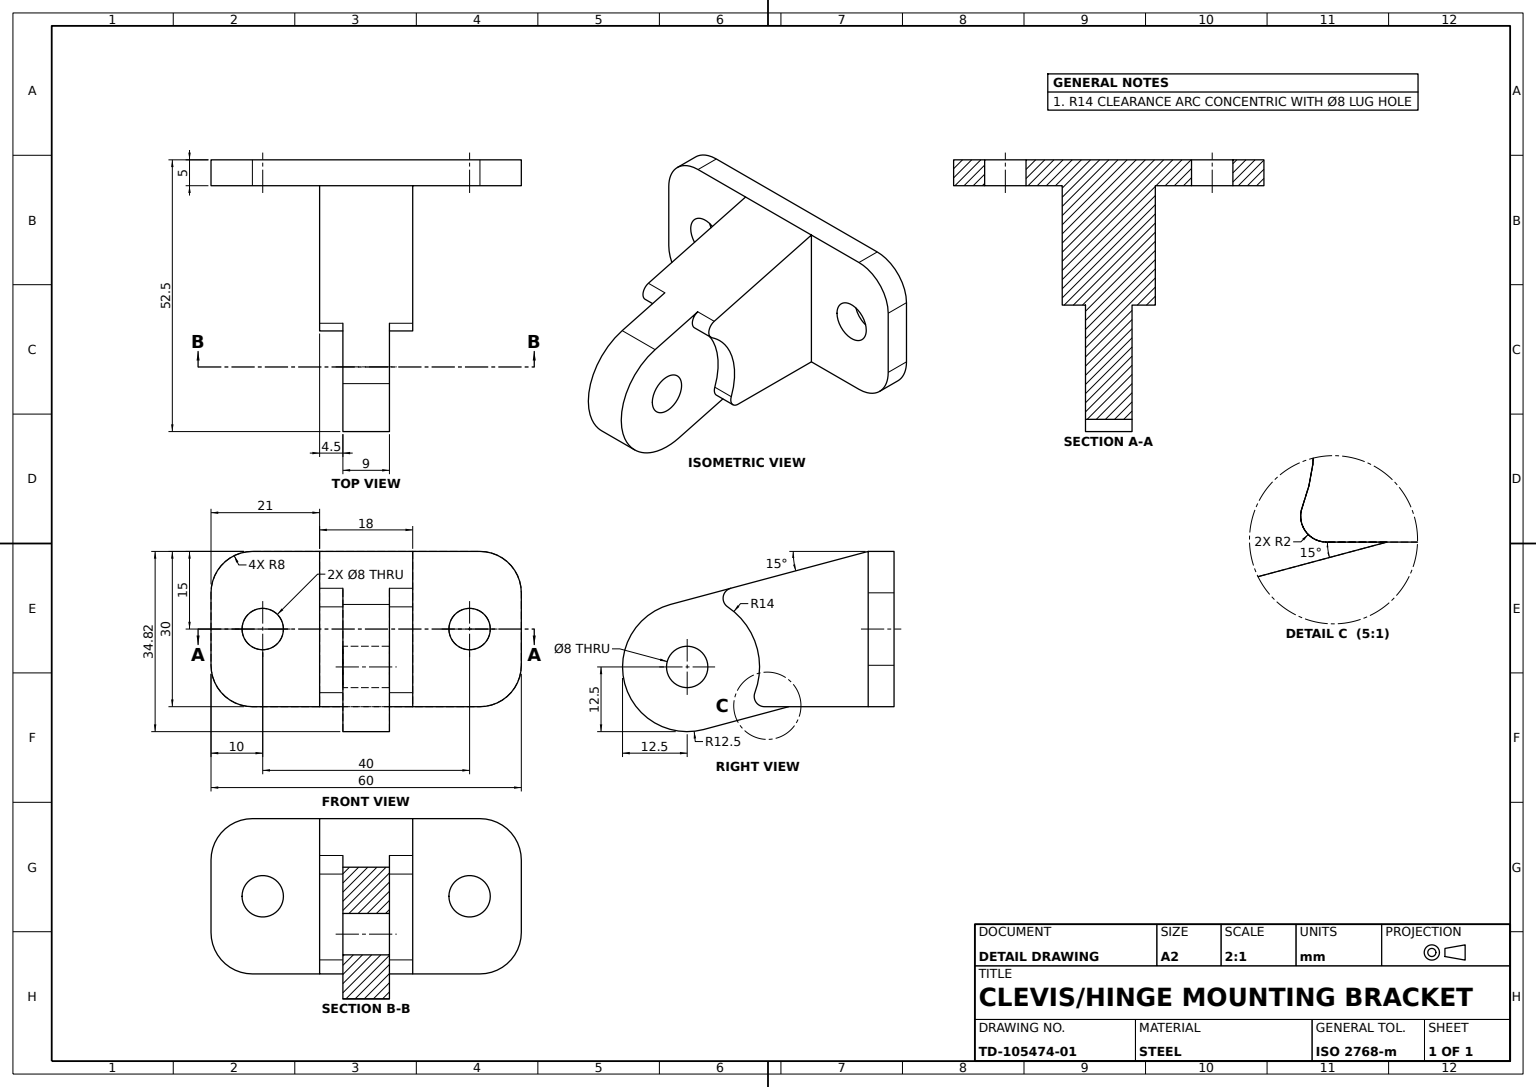
from build123d import *

# Parameters (mm, degrees)
BASE_PLATE_SKETCH_R   = 4
BASE_PLATE_DEPTH      = 5
LUG_PROFILE_SKETCH_R  = 4
LUG_SUPPORT_WEB_DEPTH = 4.5
LUG_EYE_DEPTH         = 9


with BuildPart() as part:
    # Base Plate Sketch → Base Plate (new body)
    with BuildSketch(Plane.XY):
        with BuildLine():
            Line((-22, -15), (22, -15))
            ThreePointArc((22, -15), (27.656854249, -12.656854249), (30, -7))
            Line((30, -7), (30, 7))
            ThreePointArc((30, 7), (27.656854249, 12.656854249), (22, 15))
            Line((22, 15), (-22, 15))
            ThreePointArc((-22, 15), (-27.656854249, 12.656854249), (-30, 7))
            Line((-30, 7), (-30, -7))
            ThreePointArc((-30, -7), (-27.656854249, -12.656854249), (-22, -15))
        make_face()
        with Locations((20, 0)):
            Circle(BASE_PLATE_SKETCH_R, mode=Mode.SUBTRACT)
        with Locations((-20, 0)):
            Circle(BASE_PLATE_SKETCH_R, mode=Mode.SUBTRACT)
    extrude(amount=BASE_PLATE_DEPTH)



with BuildPart() as body_2:
    # Lug Profile Sketch → Lug Support Web (new, symmetric)
    with BuildSketch(Plane(origin=(0, 0, 0), x_dir=(0, 0, -1), z_dir=(1, 0, 0))):
        with BuildLine():
            ThreePointArc((-32.17423683, 4.289332839), (-33.028883618, 6.27753657), (-31.573908753, 7.87954261))
            Line((-31.573908753, 7.87954261), (-43.235238064, 4.754898838))
            ThreePointArc((-43.235238064, 4.754898838), (-52.086936749, -10.506015692), (-36.861605806, -19.418780673))
            Line((-36.861605806, -19.418780673), (-36.668125757, -19.36693785))
            Line((-36.668125757, -19.36693785), (-20.370491826, -15))
            Line((-20.370491826, -15), (-25.04245288, -15))
            ThreePointArc((-25.04245288, -15), (-26.688692003, -14.135736214), (-26.91214627, -12.289896749))
            ThreePointArc((-26.91214627, -12.289896749), (-26.655991742, -3.083912061), (-32.17423683, 4.289332839))
        make_face()
        with Locations((-40, -7.31917399)):
            Circle(LUG_PROFILE_SKETCH_R, mode=Mode.SUBTRACT)
    extrude(amount=LUG_SUPPORT_WEB_DEPTH, both=True)


with BuildPart() as part_1:
    add(part.part)

    add(body_2.part)  # Lug Eye merges body 2
    # Sketch4_3 → Lug Eye (add, symmetric)
    with BuildSketch(Plane(origin=(0, 0, 0), x_dir=(0, 0, -1), z_dir=(1, 0, 0))):
        with BuildLine():
            Line((-5, -15), (-5, 15))
            Line((-5, 15), (-31.573908753, 7.87954261))
            ThreePointArc((-31.573908753, 7.87954261), (-33.028883618, 6.27753657), (-32.17423683, 4.289332839))
            ThreePointArc((-32.17423683, 4.289332839), (-26.655991742, -3.083912061), (-26.91214627, -12.289896749))
            ThreePointArc((-26.91214627, -12.289896749), (-26.688692003, -14.135736214), (-25.04245288, -15))
            Line((-25.04245288, -15), (-20.370491826, -15))
            Line((-20.370491826, -15), (-5, -15))
        make_face()
    extrude(amount=LUG_EYE_DEPTH, both=True)


solid = part_1.part
